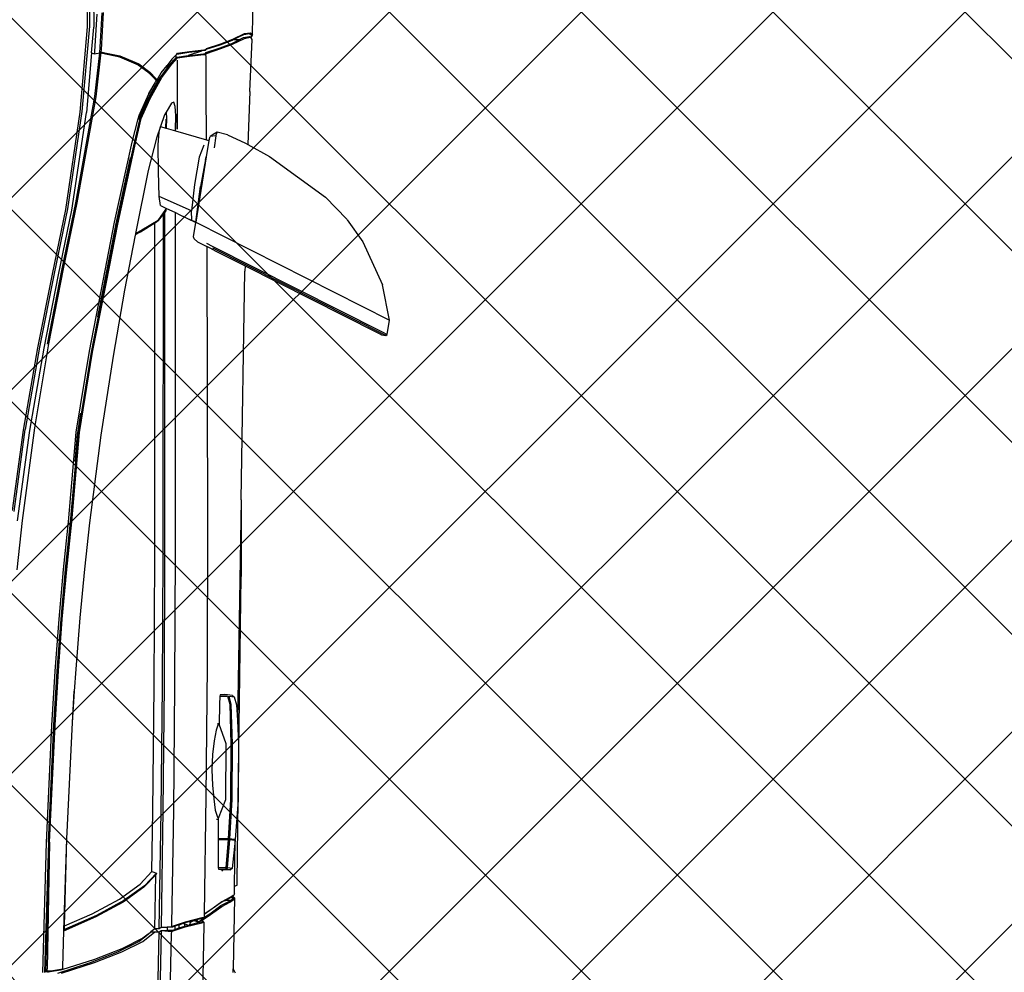
# Model space of a CAD drawing. Units: inches. Extents: x 2167 to 2589, y 1680 to 2489.
# Tile 11 of 38: x 2299 to 2335, y 1761 to 1796. Entities that reach past the tile are written whole.
import ezdxf

# ---------------------------------------------------------------- set-up
doc = ezdxf.new("R2010")
doc.units = ezdxf.units.IN
doc.header["$MEASUREMENT"] = 0
doc.layers.get('0').update_dxf_attribs({"color": 250})
doc.layers.add('C-PRKG-VEHS', color=8, linetype='Continuous', lineweight=13)
doc.layers.add('L-PVMT-PATT', color=252, linetype='Continuous', lineweight=13)
doc.layers.add('Edges', color=250, linetype='Continuous')

# ---------------------------------------------------------------- blocks, each defined once
blk = doc.blocks.new('Nissan Qashqai pl')
at = {"layer": 'Edges'}
for p, q in [((8.8918, 12.7444), (9.0186, 12.9956)), ((9.0186, 12.9956), (8.9731, 12.9865)), ((9.0374, 12.9925), (9.0186, 12.9956)), ((8.9173, 12.961), (8.9731, 12.9865)), ((9.0333, 12.9845), (8.9232, 12.7662)), ((9.0386, 12.9907), (8.9254, 12.7664)), ((9.0356, 12.9888), (9.0333, 12.9845)), ((9.0347, 12.9794), (9.0362, 12.9822)), ((9.0356, 12.9888), (9.0374, 12.9925)), ((9.0362, 12.9822), (9.037, 12.9838)), ((9.0371, 12.9841), (9.037, 12.9838)), ((9.0371, 12.9841), (9.0376, 12.985)), ((9.0376, 12.985), (9.0371, 12.9847)), ((9.0386, 12.9907), (9.0374, 12.9925)), ((9.0376, 12.985), (9.0386, 12.9907)), ((8.9483, 12.8082), (9.0343, 12.9785)), ((9.0343, 12.9785), (9.0347, 12.9794)), ((8.8885, 12.9405), (8.9173, 12.961)), ((8.8591, 12.9127), (8.8879, 12.94)), ((8.8885, 12.9405), (8.8879, 12.94)), ((8.8066, 12.84), (8.8591, 12.9127)), ((8.7908, 12.812), (8.8066, 12.84)), ((8.6489, 12.8179), (8.5719, 12.8193)), ((8.646, 12.8153), (8.6489, 12.8179)), ((8.646, 12.8153), (8.646, 12.8153)), ((8.6472, 12.8076), (8.646, 12.8153)), ((8.647, 12.8142), (8.6498, 12.8168)), ((8.6482, 12.8067), (8.647, 12.8142)), ((8.6489, 12.8179), (8.6527, 12.8156)), ((8.6498, 12.8168), (8.6524, 12.8153)), ((8.651, 12.814), (8.652, 12.815)), ((8.6524, 12.8064), (8.651, 12.814)), ((8.652, 12.815), (8.6524, 12.8153)), ((8.6534, 12.8073), (8.652, 12.815)), ((8.6524, 12.8153), (8.6527, 12.8156)), ((8.6527, 12.8156), (8.6537, 12.8167)), ((8.6547, 12.8176), (8.6537, 12.8167)), ((8.6537, 12.8167), (8.6537, 12.8166)), ((8.7222, 12.8144), (8.6547, 12.8176)), ((8.7222, 12.8144), (8.7908, 12.812)), ((8.6546, 12.7926), (8.6472, 12.8076)), ((8.655, 12.7929), (8.6482, 12.8067)), ((8.655, 12.801), (8.6524, 12.8064)), ((8.6608, 12.7921), (8.6534, 12.8073)), ((8.7785, 12.7855), (8.7891, 12.8089)), ((8.7891, 12.8089), (8.7908, 12.812)), ((8.928, 12.7679), (8.9483, 12.8082)), ((8.9483, 12.8082), (8.9552, 12.8081)), ((9.2517, 12.8031), (8.9552, 12.8081)), ((9.2517, 12.8031), (9.351, 12.803)), ((9.2517, 12.8031), (9.5372, 12.7983)), ((9.641, 12.7991), (9.351, 12.803)), ((8.6606, 12.7768), (8.6546, 12.7926)), ((8.6598, 12.7913), (8.655, 12.801)), ((8.655, 12.7929), (8.655, 12.801)), ((8.6556, 12.7918), (8.655, 12.7929)), ((8.655, 12.7922), (8.655, 12.7929)), ((8.6616, 12.7758), (8.6556, 12.7918)), ((8.6657, 12.7758), (8.6598, 12.7913)), ((8.6667, 12.7767), (8.6608, 12.7921)), ((9.5052, 12.7918), (9.5044, 12.7856)), ((9.5052, 12.7918), (9.5069, 12.7941)), ((9.5061, 12.7878), (9.5069, 12.7941)), ((9.5168, 12.7904), (9.5061, 12.7878)), ((9.5069, 12.7941), (9.5176, 12.7972)), ((9.5167, 12.7883), (9.5679, 12.7899)), ((9.5679, 12.792), (9.5168, 12.7904)), ((9.5176, 12.7972), (9.5372, 12.7983)), ((9.5372, 12.7983), (9.5689, 12.7999)), ((9.6401, 12.7914), (9.5679, 12.792)), ((9.5679, 12.7899), (9.64, 12.7892)), ((9.5689, 12.7999), (9.641, 12.7991)), ((9.64, 12.7892), (9.6912, 12.7865)), ((9.6913, 12.7886), (9.6401, 12.7914)), ((9.641, 12.7991), (9.6921, 12.7956)), ((9.7466, 12.7978), (9.641, 12.7991)), ((9.6913, 12.7886), (9.6912, 12.7865)), ((9.692, 12.7943), (9.6913, 12.7886)), ((9.6921, 12.7956), (9.692, 12.7943)), ((9.6922, 12.7943), (9.692, 12.7943)), ((9.6922, 12.7943), (9.6921, 12.7956)), ((9.7526, 12.7946), (9.6921, 12.7956)), ((9.6922, 12.7885), (9.6921, 12.7864)), ((9.6922, 12.7885), (9.693, 12.7955)), ((9.6922, 12.7885), (9.6922, 12.7943)), ((9.7288, 12.7854), (9.6922, 12.7885)), ((9.693, 12.7955), (9.7296, 12.7914)), ((9.7296, 12.7914), (9.7288, 12.7854)), ((9.7296, 12.7914), (9.7314, 12.7895)), ((9.7306, 12.7834), (9.7314, 12.7895)), ((9.7314, 12.7895), (9.7313, 12.7798)), ((9.7511, 12.7979), (9.7466, 12.7978)), ((9.7526, 12.7946), (9.7511, 12.7979)), ((9.7623, 12.7945), (9.7526, 12.7946)), ((9.7623, 12.7945), (9.7643, 12.7937)), ((9.7643, 12.7937), (9.7652, 12.7927)), ((9.7643, 12.7937), (9.7648, 12.7929)), ((9.7648, 12.7929), (9.7648, 12.7929)), ((9.7648, 12.7929), (9.7664, 12.7902)), ((9.7652, 12.7927), (9.7665, 12.7907)), ((9.7665, 12.7904), (9.7664, 12.7902)), ((9.7664, 12.7902), (9.7674, 12.7885)), ((9.7667, 12.7933), (9.7665, 12.7907)), ((9.7665, 12.7907), (9.7676, 12.7889)), ((9.7677, 12.7944), (9.7667, 12.7933)), ((9.7676, 12.7931), (9.7667, 12.7933)), ((9.7673, 12.7899), (9.7676, 12.7931)), ((9.7673, 12.7897), (9.7673, 12.7899)), ((9.7673, 12.7897), (9.7676, 12.7889)), ((9.7674, 12.7885), (9.7728, 12.7781)), ((9.769, 12.7926), (9.7676, 12.7931)), ((9.7676, 12.7889), (9.7684, 12.7875)), ((9.7676, 12.7887), (9.7678, 12.7882)), ((9.7677, 12.7944), (9.7677, 12.7944)), ((9.77, 12.7936), (9.7677, 12.7944)), ((9.7677, 12.7944), (9.8598, 12.7928)), ((9.7712, 12.7892), (9.769, 12.7926)), ((9.7734, 12.7884), (9.77, 12.7936)), ((9.7707, 12.7848), (9.7709, 12.7893)), ((9.7709, 12.7893), (9.7712, 12.7892)), ((9.7724, 12.7874), (9.7712, 12.7892)), ((9.8598, 12.7928), (9.8614, 12.7937)), ((9.8643, 12.7927), (9.8598, 12.7928)), ((9.8614, 12.7937), (9.8647, 12.7956)), ((8.6667, 12.7584), (8.6606, 12.7768)), ((8.6675, 12.758), (8.6616, 12.7758)), ((8.6718, 12.7574), (8.6657, 12.7758)), ((8.6728, 12.7584), (8.6667, 12.7767)), ((8.7785, 12.7855), (8.7751, 12.7719)), ((9.5037, 12.7806), (9.5045, 12.7814)), ((9.5044, 12.7856), (9.5045, 12.7814)), ((9.5045, 12.7814), (9.5045, 12.7759)), ((9.5045, 12.7759), (9.5063, 12.7755)), ((9.5061, 12.7856), (9.5167, 12.7883)), ((9.5063, 12.7755), (9.5061, 12.7856)), ((9.5678, 12.7837), (9.5426, 12.7747)), ((9.64, 12.7831), (9.5678, 12.7837)), ((9.6645, 12.7737), (9.64, 12.7831)), ((9.6912, 12.7811), (9.6911, 12.7796)), ((9.6911, 12.7796), (9.6911, 12.7732)), ((9.6912, 12.7865), (9.6912, 12.7811)), ((9.692, 12.7811), (9.6912, 12.7811)), ((9.692, 12.7811), (9.6921, 12.7864)), ((9.692, 12.7796), (9.692, 12.7811)), ((9.692, 12.7733), (9.692, 12.7796)), ((9.6921, 12.7864), (9.7288, 12.7832)), ((9.7288, 12.7832), (9.7287, 12.7734)), ((9.7306, 12.7834), (9.7288, 12.7854)), ((9.7288, 12.7854), (9.7288, 12.7832)), ((9.7288, 12.7832), (9.7306, 12.7834)), ((9.7305, 12.7738), (9.7306, 12.7834)), ((9.7305, 12.7738), (9.7313, 12.7798)), ((9.733, 12.7782), (9.7313, 12.7798)), ((9.7684, 12.7875), (9.7717, 12.781)), ((9.7717, 12.781), (9.7707, 12.7848)), ((9.7717, 12.781), (9.7738, 12.7771)), ((9.7778, 12.777), (9.7724, 12.7874)), ((9.7728, 12.7781), (9.7832, 12.7637)), ((9.7788, 12.778), (9.7734, 12.7884)), ((9.7738, 12.7771), (9.7842, 12.7627)), ((9.7883, 12.7626), (9.7778, 12.777)), ((9.7894, 12.7636), (9.7788, 12.778)), ((8.7751, 12.7719), (8.7779, 12.7668)), ((8.7798, 12.7703), (8.7751, 12.7719)), ((8.7779, 12.7668), (8.7807, 12.763)), ((8.7798, 12.7703), (8.7807, 12.763)), ((8.7798, 12.7703), (8.7954, 12.7683)), ((8.7849, 12.7615), (8.7807, 12.763)), ((8.9232, 12.7662), (8.9194, 12.7588)), ((8.928, 12.7679), (8.925, 12.762)), ((9.5063, 12.7755), (9.5168, 12.7751)), ((9.5168, 12.7751), (9.5423, 12.7746)), ((9.5423, 12.7746), (9.5422, 12.7736)), ((9.5422, 12.7736), (9.5422, 12.7725)), ((9.5422, 12.7736), (9.5424, 12.7735)), ((9.5426, 12.7747), (9.5423, 12.7746)), ((9.5426, 12.7747), (9.5424, 12.7735)), ((9.5424, 12.7735), (9.5503, 12.7706)), ((9.5503, 12.7706), (9.5641, 12.7681)), ((9.5641, 12.7681), (9.5818, 12.766)), ((9.5818, 12.766), (9.6016, 12.7651)), ((9.6016, 12.7651), (9.6215, 12.766)), ((9.6215, 12.766), (9.6395, 12.7676)), ((9.6395, 12.7676), (9.654, 12.7697)), ((9.654, 12.7697), (9.6633, 12.7726)), ((9.6633, 12.7726), (9.6645, 12.7737)), ((9.6655, 12.7733), (9.6645, 12.7737)), ((9.6655, 12.7733), (9.6911, 12.7732)), ((9.6655, 12.7713), (9.6655, 12.7733)), ((9.6911, 12.7732), (9.692, 12.7733)), ((9.692, 12.7733), (9.7287, 12.7734)), ((9.7287, 12.7734), (9.7305, 12.7738)), ((9.7832, 12.7637), (9.7887, 12.7552)), ((9.7965, 12.7526), (9.7894, 12.7636)), ((8.6675, 12.758), (8.6667, 12.7584)), ((8.6679, 12.7578), (8.6675, 12.758)), ((8.6676, 12.7576), (8.6675, 12.7576)), ((8.6675, 12.7576), (8.6675, 12.7576)), ((8.6675, 12.7576), (8.6676, 12.7576)), ((8.6676, 12.7576), (8.6677, 12.7576)), ((8.6677, 12.7576), (8.6677, 12.7576)), ((8.6677, 12.7576), (8.6682, 12.7576)), ((8.6682, 12.7576), (8.6679, 12.7578)), ((8.6682, 12.7576), (8.6692, 12.7566)), ((8.6682, 12.7572), (8.6682, 12.7576)), ((8.6684, 12.7554), (8.6682, 12.7572)), ((8.6682, 12.7572), (8.6692, 12.7566)), ((8.6684, 12.7554), (8.6685, 12.7549)), ((8.6684, 12.755), (8.6684, 12.7554)), ((8.6703, 12.7361), (8.6684, 12.755)), ((8.6692, 12.7566), (8.6697, 12.7519)), ((8.6697, 12.7519), (8.6698, 12.7516)), ((8.6714, 12.7353), (8.6697, 12.7519)), ((8.6698, 12.7516), (8.6755, 12.7343)), ((8.6729, 12.7568), (8.6718, 12.7574)), ((8.674, 12.7578), (8.6728, 12.7584)), ((8.6733, 12.7566), (8.6729, 12.7568)), ((8.6735, 12.7544), (8.6733, 12.7566)), ((8.6754, 12.7353), (8.6735, 12.7544)), ((8.6742, 12.7576), (8.674, 12.7578)), ((8.6742, 12.7584), (8.6743, 12.7582)), ((8.6744, 12.755), (8.6742, 12.7576)), ((8.6744, 12.7576), (8.6742, 12.7576)), ((8.6744, 12.7578), (8.6744, 12.7576)), ((8.6773, 12.7577), (8.6744, 12.7576)), ((8.6764, 12.736), (8.6744, 12.755)), ((8.6791, 12.7578), (8.677, 12.7578)), ((8.6791, 12.7577), (8.6773, 12.7577)), ((8.7205, 12.7579), (8.6791, 12.7578)), ((8.6791, 12.7577), (8.6791, 12.7578)), ((8.6878, 12.7577), (8.6791, 12.7578)), ((8.6878, 12.7577), (8.6791, 12.7577)), ((8.6878, 12.7577), (8.6878, 12.7577)), ((8.6911, 12.7577), (8.6878, 12.7577)), ((8.7205, 12.7579), (8.6911, 12.7577)), ((8.7849, 12.7582), (8.7205, 12.7579)), ((8.7734, 12.7181), (8.7849, 12.7582)), ((8.7849, 12.7615), (8.7858, 12.7613)), ((8.7849, 12.7582), (8.7856, 12.7608)), ((8.7858, 12.7613), (8.7856, 12.7608)), ((8.7858, 12.7613), (8.807, 12.758)), ((8.7917, 12.7547), (8.8075, 12.7486)), ((8.8102, 12.7568), (8.807, 12.758)), ((8.807, 12.758), (8.8918, 12.7444)), ((8.8102, 12.7568), (8.8455, 12.7506)), ((8.8918, 12.7444), (8.8455, 12.7506)), ((8.9171, 12.7464), (8.9233, 12.7586)), ((8.925, 12.762), (8.9233, 12.7586)), ((8.9233, 12.7586), (9.2886, 12.7594)), ((9.2886, 12.7594), (9.4673, 12.7589)), ((9.4673, 12.7589), (9.6358, 12.7575)), ((9.6358, 12.7575), (9.7887, 12.7552)), ((9.7842, 12.7627), (9.7891, 12.7552)), ((9.7933, 12.7549), (9.7883, 12.7626)), ((9.7887, 12.7552), (9.7891, 12.7552)), ((9.7891, 12.7552), (9.79, 12.7552)), ((9.79, 12.7552), (9.7931, 12.7552)), ((9.7931, 12.7552), (9.7934, 12.7535)), ((9.7931, 12.7552), (9.7933, 12.7549)), ((9.7933, 12.7549), (9.7941, 12.7541)), ((9.7934, 12.7535), (9.7938, 12.7538)), ((9.7934, 12.7535), (9.7937, 12.7524)), ((9.7937, 12.7524), (9.7992, 12.7308)), ((9.7941, 12.7541), (9.7943, 12.7535)), ((9.7955, 12.7516), (9.7943, 12.7535)), ((9.7943, 12.7535), (9.7964, 12.7453)), ((9.7963, 12.7523), (9.7955, 12.7516)), ((9.7963, 12.7523), (9.7963, 12.7524)), ((9.7964, 12.7524), (9.7963, 12.7523)), ((9.7992, 12.7476), (9.7963, 12.7523)), ((9.7967, 12.7526), (9.7964, 12.7524)), ((9.7964, 12.7525), (9.7964, 12.7524)), ((9.7964, 12.7524), (9.7996, 12.7475)), ((9.7983, 12.7541), (9.7965, 12.7526)), ((9.7965, 12.7526), (9.7967, 12.7526)), ((9.7977, 12.7535), (9.7967, 12.7526)), ((9.7967, 12.7526), (9.7986, 12.7526)), ((9.7982, 12.754), (9.7977, 12.7535)), ((9.7983, 12.7541), (9.7982, 12.754)), ((9.7986, 12.7526), (9.7982, 12.754)), ((9.7986, 12.7544), (9.7983, 12.7541)), ((9.7993, 12.755), (9.7986, 12.7544)), ((9.7988, 12.7516), (9.7986, 12.7526)), ((9.7998, 12.7477), (9.7988, 12.7516)), ((9.7999, 12.7522), (9.7993, 12.755)), ((9.7993, 12.755), (9.8024, 12.7549)), ((9.8054, 12.7307), (9.7999, 12.7522)), ((9.8024, 12.7549), (9.9426, 12.7518)), ((8.8075, 12.7486), (8.8429, 12.7426)), ((8.8429, 12.7426), (8.8771, 12.7388)), ((8.8771, 12.7388), (8.8585, 12.6969)), ((8.8895, 12.7393), (8.8771, 12.7388)), ((8.8815, 12.7228), (8.892, 12.7444)), ((8.8815, 12.7228), (8.8895, 12.7393)), ((8.8908, 12.7421), (8.8895, 12.7393)), ((8.8906, 12.7418), (8.8895, 12.7393)), ((8.8906, 12.7418), (8.8911, 12.7428)), ((8.892, 12.7444), (8.8908, 12.7421)), ((8.8911, 12.7428), (8.8919, 12.7444)), ((8.8911, 12.7428), (8.8919, 12.7444)), ((8.8919, 12.7444), (8.8911, 12.7428)), ((8.8919, 12.7444), (8.8918, 12.7444)), ((8.892, 12.7444), (8.8919, 12.7444)), ((8.8919, 12.7444), (8.8919, 12.7444)), ((8.8919, 12.7444), (8.8919, 12.7444)), ((8.9106, 12.7413), (8.892, 12.7444)), ((8.892, 12.7444), (8.892, 12.7444)), ((8.9131, 12.7421), (8.9106, 12.7413)), ((8.9171, 12.7464), (8.9131, 12.7421)), ((8.9171, 12.7464), (8.917, 12.7468)), ((9.7964, 12.7453), (9.7992, 12.7476)), ((9.7964, 12.7453), (9.7973, 12.7418)), ((9.7977, 12.7431), (9.7973, 12.7418)), ((9.7973, 12.7418), (9.7977, 12.7409)), ((9.7973, 12.7418), (9.7977, 12.7399)), ((9.7977, 12.7444), (9.7985, 12.7451)), ((9.7985, 12.7451), (9.7977, 12.7431)), ((9.7977, 12.7431), (9.7977, 12.7444)), ((9.7977, 12.7399), (9.7977, 12.7409)), ((9.7977, 12.7409), (9.7987, 12.7388)), ((9.7977, 12.7399), (9.7978, 12.7397)), ((9.7987, 12.7388), (9.7978, 12.7397)), ((9.7978, 12.7397), (9.7987, 12.7362)), ((9.7989, 12.7461), (9.7985, 12.7451)), ((9.7987, 12.7388), (9.7992, 12.7377)), ((9.7987, 12.7362), (9.7992, 12.7377)), ((9.7998, 12.7466), (9.7989, 12.7461)), ((9.7998, 12.7466), (9.7992, 12.7476)), ((9.7992, 12.7377), (9.8027, 12.7364)), ((9.7996, 12.7475), (9.7998, 12.7477)), ((9.8002, 12.7461), (9.7996, 12.7475)), ((9.8001, 12.7468), (9.7996, 12.7475)), ((9.8001, 12.7468), (9.7998, 12.7477)), ((9.8003, 12.7458), (9.7998, 12.7466)), ((9.8002, 12.7461), (9.8001, 12.7468)), ((9.8003, 12.7458), (9.8002, 12.7461)), ((9.8027, 12.7364), (9.8003, 12.7458)), ((8.6727, 12.7207), (8.6703, 12.7361)), ((8.6737, 12.7197), (8.6714, 12.7353)), ((8.6755, 12.7343), (8.6754, 12.7353)), ((8.6777, 12.7196), (8.6755, 12.7343)), ((8.6764, 12.7359), (8.6764, 12.736)), ((8.6788, 12.7205), (8.6764, 12.7359)), ((9.7987, 12.7362), (9.8002, 12.7301)), ((9.7992, 12.7308), (9.8044, 12.7151)), ((9.8002, 12.7301), (9.8008, 12.7285)), ((9.8008, 12.7285), (9.8014, 12.7303)), ((9.8008, 12.7285), (9.8014, 12.7265)), ((9.8014, 12.7303), (9.8031, 12.7349)), ((9.8043, 12.7303), (9.8014, 12.7303)), ((9.8014, 12.7265), (9.803, 12.723)), ((9.8014, 12.7265), (9.8026, 12.723)), ((9.8031, 12.7349), (9.8027, 12.7364)), ((9.8043, 12.7303), (9.8031, 12.7349)), ((9.8044, 12.73), (9.8043, 12.7303)), ((9.8067, 12.7229), (9.8044, 12.73)), ((9.8106, 12.715), (9.8054, 12.7307)), ((8.6737, 12.7197), (8.6727, 12.7207)), ((8.6746, 12.7189), (8.6737, 12.7197)), ((8.6785, 12.7189), (8.6746, 12.7189)), ((8.6805, 12.7132), (8.6746, 12.7189)), ((8.6785, 12.7189), (8.6777, 12.7196)), ((8.6815, 12.7162), (8.6785, 12.7189)), ((8.687, 12.7132), (8.6788, 12.7205)), ((8.6805, 12.7132), (8.6884, 12.7071)), ((8.6815, 12.7162), (8.6818, 12.7154)), ((8.6817, 12.716), (8.6815, 12.7162)), ((8.6817, 12.716), (8.6818, 12.7154)), ((8.6859, 12.7122), (8.6817, 12.716)), ((8.6818, 12.7204), (8.7012, 12.7203)), ((8.6818, 12.7154), (8.6902, 12.7081)), ((8.6927, 12.7071), (8.6859, 12.7122)), ((8.7042, 12.7002), (8.687, 12.7132)), ((8.7012, 12.7203), (8.7012, 12.7203)), ((8.7012, 12.7203), (8.7026, 12.7203)), ((8.7026, 12.7203), (8.7026, 12.7203)), ((8.7026, 12.7203), (8.7072, 12.7203)), ((8.7072, 12.7203), (8.7072, 12.7203)), ((8.7072, 12.7203), (8.7273, 12.7202)), ((8.7273, 12.7202), (8.7273, 12.7201)), ((8.7273, 12.7202), (8.7354, 12.7202)), ((8.7354, 12.7201), (8.7354, 12.7202)), ((8.7354, 12.7202), (8.742, 12.7202)), ((8.7415, 12.7177), (8.7361, 12.7158)), ((8.7361, 12.7158), (8.7373, 12.7128)), ((8.7373, 12.7128), (8.7492, 12.7059)), ((8.7534, 12.7185), (8.7415, 12.7177)), ((8.742, 12.7201), (8.742, 12.7202)), ((8.742, 12.7202), (8.742, 12.7201)), ((8.742, 12.7202), (8.742, 12.7202)), ((8.742, 12.7202), (8.7426, 12.7202)), ((8.7426, 12.7201), (8.7426, 12.7202)), ((8.7426, 12.7202), (8.7433, 12.7202)), ((8.7433, 12.7201), (8.7433, 12.7202)), ((8.7433, 12.7202), (8.7711, 12.7201)), ((8.7711, 12.7201), (8.7516, 12.72)), ((8.7718, 12.7181), (8.7534, 12.7185)), ((8.7698, 12.7058), (8.7734, 12.7181)), ((8.7734, 12.7181), (8.7718, 12.7181)), ((8.8734, 12.7057), (8.8793, 12.7181)), ((8.8793, 12.7181), (8.8815, 12.7228)), ((9.3194, 12.7179), (8.8793, 12.7181)), ((9.4919, 12.7173), (9.3194, 12.7179)), ((9.6538, 12.7157), (9.4919, 12.7173)), ((9.802, 12.7133), (9.6538, 12.7157)), ((9.8051, 12.7132), (9.802, 12.7133)), ((9.803, 12.723), (9.8026, 12.723)), ((9.8026, 12.723), (9.8046, 12.7171)), ((9.8067, 12.7229), (9.803, 12.723)), ((9.8044, 12.7151), (9.8051, 12.7132)), ((9.8046, 12.7171), (9.8086, 12.7171)), ((9.8046, 12.7171), (9.8055, 12.7143)), ((9.8061, 12.6994), (9.8051, 12.7132)), ((9.8055, 12.7143), (9.8058, 12.7073)), ((9.8086, 12.7171), (9.8067, 12.7229)), ((9.8096, 12.7142), (9.8086, 12.7171)), ((9.8098, 12.7073), (9.8096, 12.7142)), ((9.8101, 12.6993), (9.8112, 12.7131)), ((9.8112, 12.7131), (9.8106, 12.715)), ((9.8143, 12.713), (9.8112, 12.7131)), ((9.9414, 12.71), (9.8143, 12.713)), ((8.6917, 12.7071), (8.6884, 12.7071)), ((8.698, 12.6996), (8.6884, 12.7071)), ((8.6902, 12.7081), (8.6917, 12.7071)), ((8.6917, 12.7071), (8.7075, 12.6955)), ((8.6927, 12.7071), (8.6923, 12.7071)), ((8.7032, 12.6992), (8.6927, 12.7071)), ((8.7071, 12.6942), (8.698, 12.6996)), ((8.7302, 12.684), (8.7032, 12.6992)), ((8.7312, 12.6851), (8.7042, 12.7002)), ((8.7492, 12.7059), (8.7572, 12.7062)), ((8.7492, 12.7059), (8.7524, 12.704)), ((8.7524, 12.704), (8.7828, 12.6934)), ((8.7572, 12.7062), (8.7698, 12.7058)), ((8.7698, 12.7057), (8.7583, 12.706)), ((8.7678, 12.6988), (8.7698, 12.7057)), ((8.7698, 12.7057), (8.7698, 12.7058)), ((8.87, 12.6987), (8.8734, 12.7057)), ((8.8734, 12.7057), (8.8768, 12.7057)), ((8.8751, 12.7054), (8.8768, 12.7057)), ((8.8893, 12.6956), (8.8751, 12.7054)), ((8.8768, 12.7057), (8.879, 12.704)), ((8.879, 12.704), (9.3198, 12.7039)), ((8.879, 12.704), (8.881, 12.7023)), ((9.3225, 12.7021), (8.881, 12.7023)), ((8.881, 12.7023), (8.8893, 12.6956)), ((9.3198, 12.7039), (9.4922, 12.7033)), ((9.4936, 12.7013), (9.3225, 12.7021)), ((9.4922, 12.7033), (9.654, 12.7018)), ((9.6552, 12.6997), (9.4936, 12.7013)), ((9.654, 12.7018), (9.8061, 12.6994)), ((9.8078, 12.6971), (9.6552, 12.6997)), ((9.8058, 12.7073), (9.8098, 12.7073)), ((9.8058, 12.7073), (9.8061, 12.6994)), ((9.8061, 12.6994), (9.8078, 12.6971)), ((9.8101, 12.6993), (9.8098, 12.7073)), ((9.8119, 12.697), (9.8101, 12.6993)), ((9.8101, 12.6993), (9.9411, 12.6966)), ((8.697, 12.685), (8.7055, 12.6927)), ((8.6979, 12.6839), (8.7062, 12.6915)), ((8.7062, 12.6915), (8.6987, 12.6845)), ((8.7055, 12.6927), (8.7071, 12.6942)), ((8.7062, 12.6915), (8.7067, 12.6919)), ((8.7067, 12.6919), (8.7083, 12.6934)), ((8.7071, 12.6942), (8.7083, 12.6934)), ((8.7075, 12.6955), (8.7346, 12.6806)), ((8.7083, 12.6934), (8.7083, 12.6934)), ((8.7083, 12.6934), (8.7083, 12.6934)), ((8.7102, 12.6923), (8.7083, 12.6934)), ((8.7083, 12.6934), (8.7083, 12.6934)), ((8.7108, 12.6919), (8.7102, 12.6923)), ((8.7102, 12.6923), (8.7102, 12.6923)), ((8.7257, 12.6833), (8.7108, 12.6919)), ((8.7248, 12.6836), (8.7108, 12.6919)), ((8.7748, 12.6967), (8.7678, 12.6988)), ((8.7916, 12.6954), (8.7748, 12.6967)), ((8.7828, 12.6934), (8.8245, 12.6828)), ((8.8259, 12.6959), (8.7916, 12.6954)), ((8.8585, 12.6969), (8.8259, 12.6959)), ((8.87, 12.6987), (8.8585, 12.6969)), ((8.8893, 12.6956), (8.9021, 12.6745)), ((8.8913, 12.6936), (8.8893, 12.6956)), ((8.8927, 12.6913), (8.8913, 12.6936)), ((9.3224, 12.6911), (8.8927, 12.6913)), ((8.9041, 12.6725), (8.8927, 12.6913)), ((9.3225, 12.6911), (9.3224, 12.6911)), ((9.4936, 12.6904), (9.3225, 12.6911)), ((9.6552, 12.6888), (9.4936, 12.6904)), ((9.7337, 12.6875), (9.6552, 12.6888)), ((9.7337, 12.6875), (9.7357, 12.6935)), ((9.7499, 12.6721), (9.7337, 12.6875)), ((9.7357, 12.6935), (9.7378, 12.6924)), ((9.7357, 12.6935), (9.7519, 12.678)), ((9.7378, 12.6924), (9.754, 12.677)), ((9.8078, 12.6913), (9.7378, 12.6924)), ((9.8078, 12.6971), (9.8078, 12.6913)), ((9.8078, 12.6913), (9.8119, 12.6862)), ((9.9393, 12.6944), (9.8119, 12.697)), ((9.8119, 12.6912), (9.8119, 12.697)), ((9.8241, 12.6756), (9.8119, 12.6912)), ((9.8119, 12.6862), (9.8119, 12.6912)), ((8.6864, 12.6706), (8.697, 12.685)), ((8.6875, 12.6698), (8.6979, 12.6839)), ((8.6924, 12.676), (8.6883, 12.6704)), ((8.6987, 12.6845), (8.6924, 12.676)), ((8.6924, 12.676), (8.6924, 12.6762)), ((8.7257, 12.6833), (8.7248, 12.6836)), ((8.7257, 12.6832), (8.7257, 12.6833)), ((8.7257, 12.6832), (8.7508, 12.672)), ((8.7529, 12.6741), (8.7302, 12.684)), ((8.7574, 12.6737), (8.7312, 12.6851)), ((8.7346, 12.6806), (8.7491, 12.6738)), ((8.7346, 12.6806), (8.7577, 12.6709)), ((8.7508, 12.672), (8.7491, 12.6738)), ((8.7491, 12.6738), (8.7576, 12.6699)), ((8.7529, 12.6741), (8.7577, 12.6709)), ((8.757, 12.6724), (8.7529, 12.6741)), ((8.7931, 12.6653), (8.7574, 12.6737)), ((8.8245, 12.6828), (8.9063, 12.6663)), ((8.9021, 12.6745), (8.9063, 12.6663)), ((9.7519, 12.678), (9.7713, 12.6512)), ((9.754, 12.677), (9.7733, 12.6502)), ((9.8147, 12.6826), (9.8119, 12.6862)), ((9.8147, 12.6826), (9.8147, 12.6826)), ((9.8147, 12.6826), (9.8201, 12.6756)), ((9.8241, 12.6706), (9.8147, 12.6826)), ((9.8201, 12.6756), (9.8338, 12.6486)), ((9.8378, 12.6485), (9.8241, 12.6756)), ((8.6759, 12.6459), (8.6864, 12.6706)), ((8.6772, 12.6454), (8.6875, 12.6698)), ((8.6883, 12.6704), (8.6777, 12.6457)), ((8.7532, 12.6708), (8.7508, 12.672)), ((8.7575, 12.6698), (8.7532, 12.6708)), ((8.7587, 12.672), (8.757, 12.6724)), ((8.7576, 12.6699), (8.7575, 12.6698)), ((8.7881, 12.6621), (8.7575, 12.6698)), ((8.7582, 12.6707), (8.7576, 12.6699)), ((8.7577, 12.6709), (8.7582, 12.6707)), ((8.759, 12.6717), (8.7582, 12.6707)), ((8.7587, 12.672), (8.759, 12.6717)), ((8.7591, 12.6719), (8.7587, 12.672)), ((8.7591, 12.6719), (8.759, 12.6717)), ((8.7925, 12.664), (8.7591, 12.6719)), ((8.8918, 12.6392), (8.7881, 12.6621)), ((8.8941, 12.6418), (8.7925, 12.664)), ((8.8942, 12.6432), (8.7931, 12.6653)), ((8.9075, 12.6661), (8.9041, 12.6725)), ((8.9063, 12.6663), (8.9075, 12.6661)), ((8.9075, 12.6661), (8.9087, 12.6658)), ((8.9087, 12.6658), (8.9797, 12.6518)), ((9.7692, 12.6453), (9.7499, 12.6721)), ((9.8378, 12.6435), (9.8241, 12.6706)), ((8.8083, 12.6591), (8.8954, 12.6403)), ((8.9797, 12.6518), (9.0656, 12.6372)), ((9.7713, 12.6512), (9.7905, 12.6158)), ((9.7733, 12.6502), (9.7925, 12.6148)), ((9.8338, 12.6486), (9.8475, 12.613)), ((9.8516, 12.6129), (9.8378, 12.6485)), ((8.6716, 12.6242), (8.6759, 12.6459)), ((8.6772, 12.6454), (8.6721, 12.6201)), ((8.6777, 12.6457), (8.6727, 12.6213)), ((8.9679, 12.6241), (8.8918, 12.6392)), ((9.0601, 12.6092), (8.8941, 12.6418)), ((8.9696, 12.6285), (8.8942, 12.6432)), ((8.8961, 12.6401), (8.9704, 12.6257)), ((9.0656, 12.6372), (9.1676, 12.6212)), ((9.7885, 12.6099), (9.7692, 12.6453)), ((9.8516, 12.6079), (9.8378, 12.6435)), ((8.6197, 12.6241), (8.6683, 12.6215)), ((8.6721, 12.6201), (8.6204, 12.6229)), ((8.671, 12.6214), (8.6716, 12.6242)), ((9.0591, 12.6065), (8.9679, 12.6241)), ((9.06, 12.6106), (8.9696, 12.6285)), ((8.9704, 12.6257), (8.9708, 12.6256)), ((8.9708, 12.6256), (9.0143, 12.6169)), ((8.5538, 12.6111), (8.6387, 12.6123)), ((8.622, 12.6161), (8.6699, 12.6132)), ((8.6721, 12.6093), (8.6387, 12.6123)), ((8.6683, 12.6215), (8.671, 12.6214)), ((8.6699, 12.6132), (8.6721, 12.613)), ((8.671, 12.6214), (8.6721, 12.6201)), ((8.6727, 12.6213), (8.6721, 12.6201)), ((8.6733, 12.6129), (8.6721, 12.6201)), ((8.7287, 12.6134), (8.6721, 12.6201)), ((8.6721, 12.6127), (8.6721, 12.613)), ((8.6721, 12.613), (8.6733, 12.6129)), ((8.6721, 12.6093), (8.6733, 12.6129)), ((8.6727, 12.6213), (8.6753, 12.621)), ((8.6753, 12.621), (8.7292, 12.6146)), ((8.8666, 12.5888), (8.7287, 12.6134)), ((8.7292, 12.6146), (8.8666, 12.5901)), ((9.1644, 12.5938), (9.06, 12.6106)), ((9.1676, 12.6212), (9.2814, 12.6065)), ((9.8039, 12.5741), (9.7885, 12.6099)), ((9.7905, 12.6158), (9.8087, 12.574)), ((9.7925, 12.6148), (9.8107, 12.573)), ((9.8475, 12.613), (9.8611, 12.5708)), ((9.8652, 12.5704), (9.8516, 12.6129)), ((8.5531, 12.6055), (8.6375, 12.6066)), ((8.5544, 12.6026), (8.6386, 12.6037)), ((8.6375, 12.6066), (8.7481, 12.5968)), ((8.6386, 12.6037), (8.7491, 12.594)), ((8.6721, 12.6093), (8.7496, 12.6025)), ((8.8761, 12.5839), (8.7496, 12.6025)), ((9.1639, 12.5895), (9.0591, 12.6065)), ((9.1645, 12.5924), (9.0601, 12.6092)), ((9.2814, 12.6065), (9.3416, 12.5999)), ((9.3416, 12.5999), (9.4048, 12.5941)), ((9.8652, 12.5654), (9.8516, 12.6079)), ((8.7481, 12.5968), (8.8745, 12.5782)), ((8.7491, 12.594), (8.8754, 12.5755)), ((8.8666, 12.5901), (8.9521, 12.5726)), ((8.9522, 12.5713), (8.8666, 12.5888)), ((9.1393, 12.5951), (9.1647, 12.591)), ((9.2801, 12.5794), (9.1639, 12.5895)), ((9.2803, 12.5836), (9.1644, 12.5938)), ((9.2804, 12.5821), (9.1645, 12.5924)), ((9.1647, 12.591), (9.1668, 12.5908)), ((9.1668, 12.5908), (9.2019, 12.5877)), ((9.4048, 12.5941), (9.471, 12.5888)), ((9.471, 12.5888), (9.4997, 12.5869)), ((9.5404, 12.5844), (9.4997, 12.5869)), ((9.4997, 12.5869), (9.5403, 12.5842)), ((9.5403, 12.5842), (9.6913, 12.5767)), ((9.6912, 12.5774), (9.5404, 12.5844)), ((8.8745, 12.5782), (8.9583, 12.5609)), ((8.8754, 12.5755), (8.9591, 12.5583)), ((8.9598, 12.5666), (8.8761, 12.5839)), ((8.9521, 12.5726), (9.0495, 12.5536)), ((9.3418, 12.5729), (9.2801, 12.5794)), ((9.3418, 12.5771), (9.2803, 12.5836)), ((9.3419, 12.5756), (9.2804, 12.5821)), ((9.4062, 12.5713), (9.3418, 12.5771)), ((9.4064, 12.5671), (9.3418, 12.5729)), ((9.4063, 12.5699), (9.3419, 12.5756)), ((9.8039, 12.5741), (9.6912, 12.5774)), ((9.6913, 12.5767), (9.8099, 12.573)), ((9.8087, 12.574), (9.8039, 12.5741)), ((9.8099, 12.573), (9.8087, 12.574)), ((9.8099, 12.573), (9.8107, 12.573)), ((9.8107, 12.573), (9.8573, 12.5716)), ((9.8573, 12.5716), (9.8603, 12.5715)), ((9.8603, 12.5715), (9.8605, 12.5696)), ((9.8611, 12.5708), (9.8603, 12.5715)), ((9.0497, 12.5523), (8.9522, 12.5713)), ((8.9583, 12.5609), (9.0538, 12.5419)), ((9.0552, 12.5477), (8.9598, 12.5666)), ((9.4735, 12.5663), (9.4062, 12.5713)), ((9.4736, 12.5648), (9.4063, 12.5699)), ((9.4739, 12.5621), (9.4064, 12.5671)), ((9.5437, 12.5619), (9.4735, 12.5663)), ((9.5438, 12.5605), (9.4736, 12.5648)), ((9.5443, 12.5579), (9.4739, 12.5621)), ((9.6953, 12.5549), (9.5437, 12.5619)), ((9.6954, 12.5535), (9.5438, 12.5605)), ((9.8605, 12.5696), (9.8626, 12.5564)), ((9.8612, 12.5707), (9.8611, 12.5708)), ((9.8612, 12.5707), (9.8615, 12.5688)), ((9.8615, 12.5688), (9.8635, 12.5556)), ((8.9591, 12.5583), (9.0546, 12.5394)), ((9.0495, 12.5536), (9.1584, 12.5351)), ((9.1617, 12.5292), (9.0552, 12.5477)), ((9.696, 12.551), (9.5443, 12.5579)), ((9.6953, 12.5549), (9.8598, 12.5517)), ((9.6953, 12.5549), (9.863, 12.5497)), ((9.6954, 12.5535), (9.8641, 12.5483)), ((9.8644, 12.5459), (9.696, 12.551)), ((9.8629, 12.5516), (9.8598, 12.5517)), ((9.8626, 12.5564), (9.8627, 12.5532)), ((9.8637, 12.5532), (9.8627, 12.5532)), ((9.8627, 12.5532), (9.8629, 12.5516)), ((9.8629, 12.5516), (9.863, 12.5497)), ((9.8641, 12.5483), (9.863, 12.5497)), ((9.8635, 12.5556), (9.8637, 12.5532)), ((9.8643, 12.5532), (9.8637, 12.5532)), ((9.8637, 12.5532), (9.8638, 12.5508)), ((9.8638, 12.5508), (9.8641, 12.5483)), ((9.0538, 12.5419), (9.1605, 12.5233)), ((9.0546, 12.5394), (9.1612, 12.5208)), ((9.1584, 12.5351), (9.2783, 12.5191)), ((9.2669, 12.5088), (9.1605, 12.5233)), ((9.1612, 12.5208), (9.2656, 12.5065)), ((9.2789, 12.5131), (9.1617, 12.5292)), ((9.2783, 12.5191), (9.3422, 12.5126))]:
    blk.add_line(p, q, dxfattribs=at)
blk = doc.blocks.new('car')
blk.add_blockref('Nissan Qashqai pl', (-9.7433, -11.9151))
blk = doc.blocks.new('carr')
blk.add_blockref('car', (0.5124, -0.007))

msp = doc.modelspace()

# ---------------------------------------------------------------- hatches: boundary and pattern name
at = {"layer": 'L-PVMT-PATT'}
h = msp.add_hatch(dxfattribs=at)
h.set_pattern_fill('ANSI37', color=256, scale=40)
h.paths.add_polyline_path([(2417.548, 1783.695), (2417.548, 1846.042), (2239.361, 1846.042), (2239.361, 1687.695), (2369.843, 1687.695), (2369.843, 1696.695), (2375.607, 1696.695), (2416.107, 1696.695), (2417.548, 1696.695)])

# ---------------------------------------------------------------- block references
at = {"layer": 'C-PRKG-VEHS', "xscale": 28.42784210623918, "yscale": 28.42784210623918, "zscale": 28.42784210623918, "rotation": 270}
msp.add_blockref('carr', (2281.736, 1778.659), dxfattribs=at)

doc.saveas('drawing.dxf')
